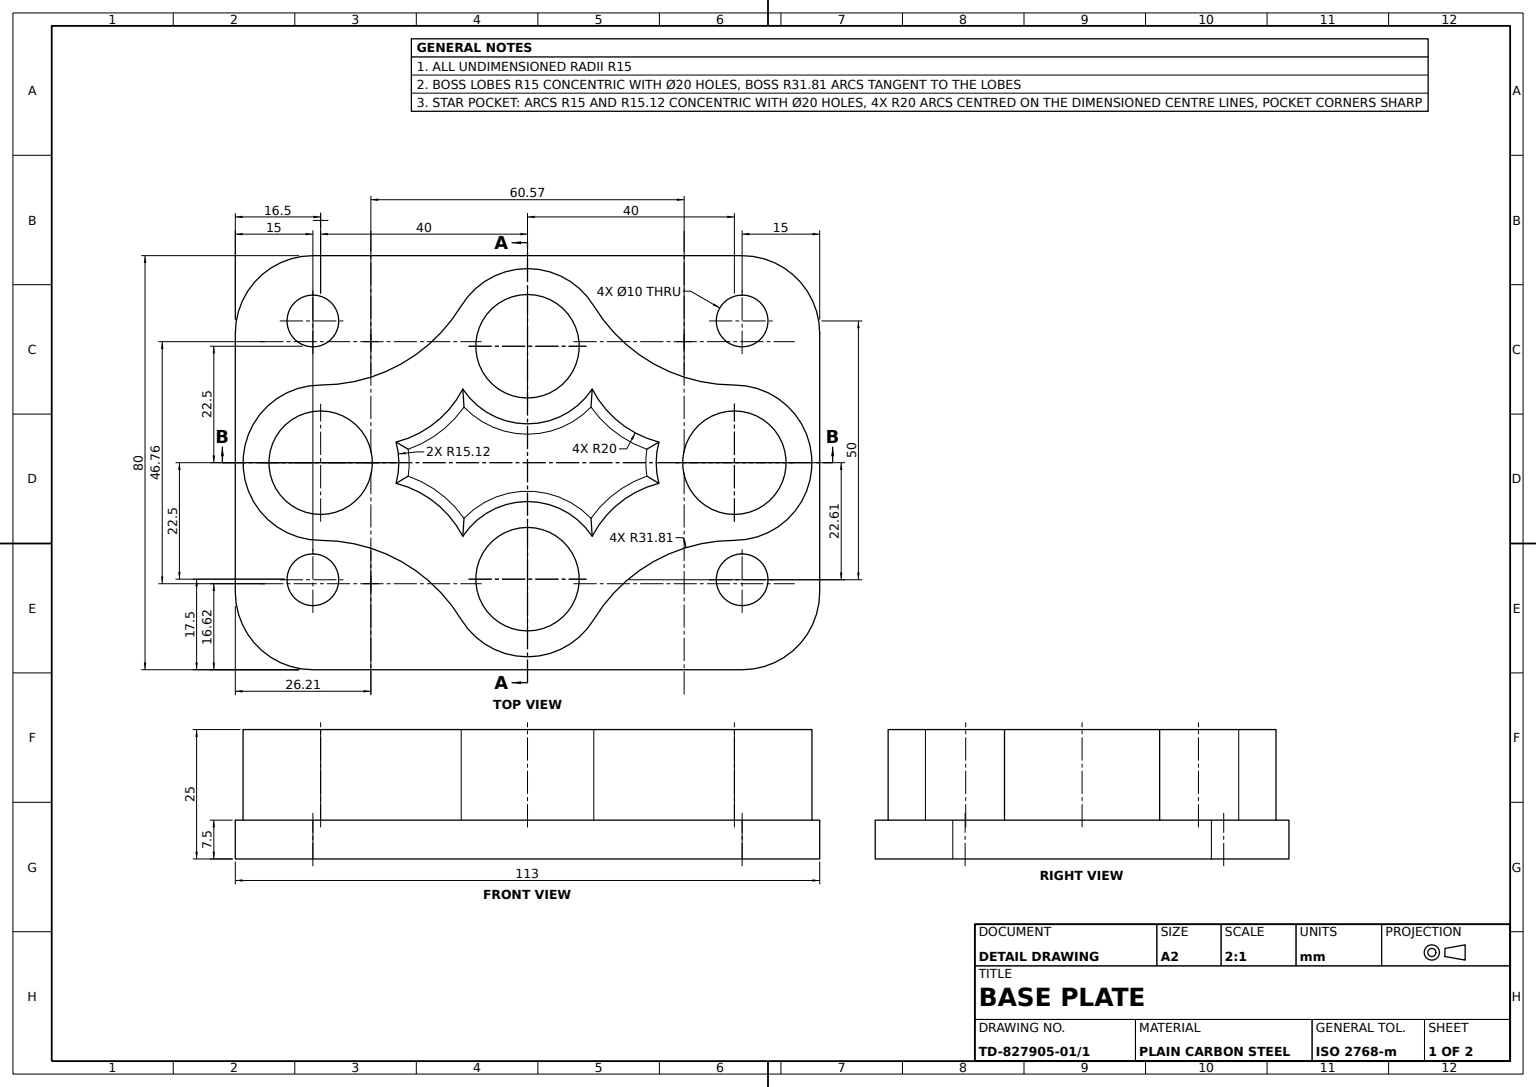
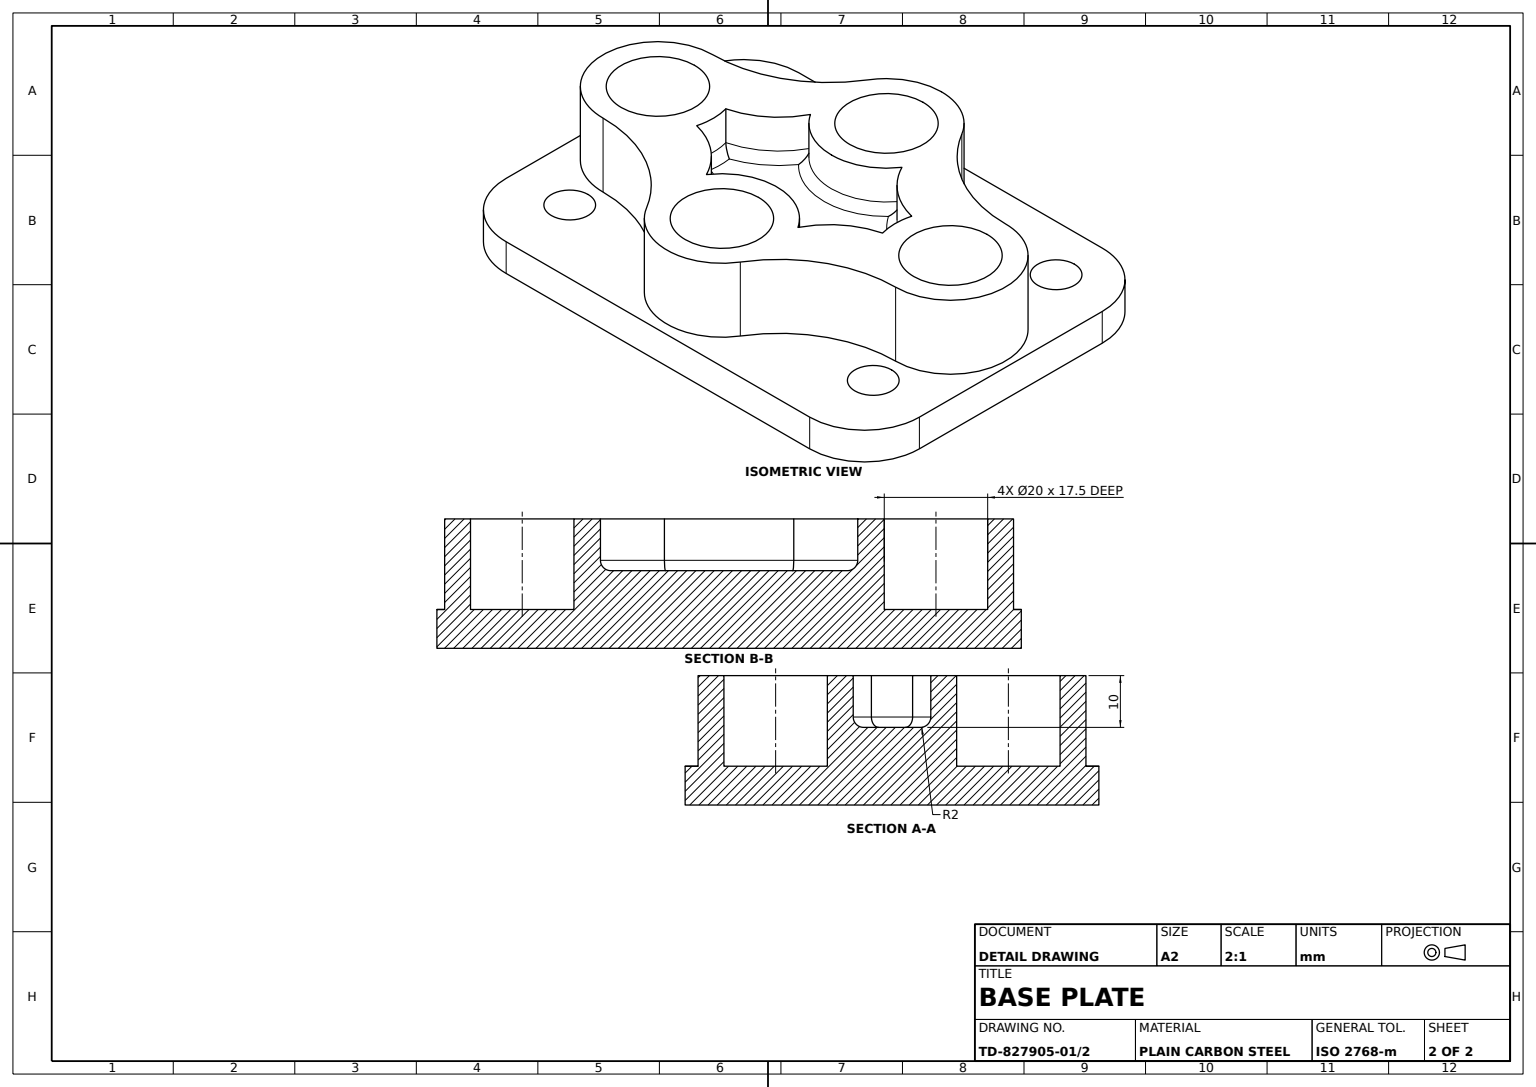
from build123d import *

# Parameters (mm, degrees)
BASE_PLATE_DEPTH           = 3.75
MOUNTING_HOLES_SKETCH_R    = 5
MOUNTING_HOLES_4X_10_DEPTH = 7.5
LOBED_BOSS_DEPTH           = 17.5
STAR_START                 = -10
STAR_POCKET_DEPTH          = 10
BOSS_BORES_SKETCH_R        = 10
BOSS_BORES_4X_DEPTH        = 17.5
POCKET_FILLETS_R2_R        = 2


with BuildPart() as part:
    # Base Plate Profile → Base Plate (new, symmetric)
    with BuildSketch(Plane(origin=(0, 0, 0), x_dir=(1, 0, 0), z_dir=(0, 1, 0))):
        with BuildLine():
            Line((41.5, -40), (-41.5, -40))
            ThreePointArc((-41.5, -40), (-52.106601718, -35.606601718), (-56.5, -25))
            Line((-56.5, -25), (-56.5, 25))
            ThreePointArc((-56.5, 25), (-52.106601718, 35.606601718), (-41.5, 40))
            Line((-41.5, 40), (41.5, 40))
            ThreePointArc((41.5, 40), (52.106601718, 35.606601718), (56.5, 25))
            Line((56.5, 25), (56.5, -25))
            ThreePointArc((56.5, -25), (52.106601718, -35.606601718), (41.5, -40))
        make_face()
    extrude(amount=BASE_PLATE_DEPTH, both=True)

    # Mounting Holes Sketch → Mounting Holes 4xØ10 (cut)
    with BuildSketch(Plane(origin=(0, 3.75, 0), x_dir=(1, 0, 0), z_dir=(0, 1, 0))):
        with Locations(Location((-41.5, 27.385128328, 0), (0, 0, 270))):
            Circle(MOUNTING_HOLES_SKETCH_R)
        with Locations(Location((-41.5, -22.614871672, 0), (0, 0, 270))):
            Circle(MOUNTING_HOLES_SKETCH_R)
        with Locations(Location((41.5, -22.614871672, 0), (0, 0, 90))):
            Circle(MOUNTING_HOLES_SKETCH_R)
        with Locations(Location((41.5, 27.385128328, 0), (0, 0, 90))):
            Circle(MOUNTING_HOLES_SKETCH_R)
    extrude(amount=-MOUNTING_HOLES_4X_10_DEPTH, mode=Mode.SUBTRACT)

    # Lobed Boss Profile → Lobed Boss (add)
    with BuildSketch(Plane(origin=(0, 3.75, 0), x_dir=(1, 0, 0), z_dir=(0, 1, 0))):
        with BuildLine():
            ThreePointArc((-40, 15), (-55, 0), (-40, -15))
            ThreePointArc((-40, -15), (-24.406968906, -19.084611389), (-12.818991098, -30.289317507))
            ThreePointArc((-12.818991098, -30.289317507), (0, -37.5), (12.818991098, -30.289317507))
            ThreePointArc((12.818991098, -30.289317507), (24.406968906, -19.084611389), (40, -15))
            ThreePointArc((40, -15), (55, 0), (40, 15))
            ThreePointArc((40, 15), (24.406968906, 19.084611389), (12.818991098, 30.289317507))
            ThreePointArc((12.818991098, 30.289317507), (0, 37.5), (-12.818991098, 30.289317507))
            ThreePointArc((-12.818991098, 30.289317507), (-24.406968906, 19.084611389), (-40, 15))
        make_face()
    extrude(amount=LOBED_BOSS_DEPTH)

    # Star Pocket Profile → Star Pocket (cut)
    with BuildSketch(Plane(origin=(0, 21.25, 0), x_dir=(1, 0, 0), z_dir=(0, 1, 0)).offset(STAR_START)):
        with BuildLine():
            ThreePointArc((-25.409734785, -3.985145132), (-24.875277829, 0), (-25.409734785, 3.985145132))
            ThreePointArc((-25.409734785, 3.985145132), (-17.85640049, 7.713077773), (-12.507806345, 14.220218576))
            ThreePointArc((-12.507806345, 14.220218576), (0, 7.5), (12.507806345, 14.220218576))
            ThreePointArc((12.507806345, 14.220218576), (17.85640049, 7.713077773), (25.409734785, 3.985145132))
            ThreePointArc((25.409734785, 3.985145132), (24.875277829, 0), (25.409734785, -3.985145132))
            ThreePointArc((25.409734785, -3.985145132), (17.85640049, -7.713077773), (12.507806345, -14.220218576))
            ThreePointArc((12.507806345, -14.220218576), (0, -7.5), (-12.507806345, -14.220218576))
            ThreePointArc((-12.507806345, -14.220218576), (-17.85640049, -7.713077773), (-25.409734785, -3.985145132))
        make_face()
    extrude(amount=STAR_POCKET_DEPTH, mode=Mode.SUBTRACT)

    # Boss Bores Sketch → Boss Bores 4x (cut)
    with BuildSketch(Plane(origin=(0, 21.25, 0), x_dir=(1, 0, 0), z_dir=(0, 1, 0))):
        with Locations(Location((40, 0, 0), (0, 0, 270))):
            Circle(BOSS_BORES_SKETCH_R)
        with Locations(Location((0, -22.5, 0), (0, 0, 270))):
            Circle(BOSS_BORES_SKETCH_R)
        with Locations(Location((0, 22.5, 0), (0, 0, 270))):
            Circle(BOSS_BORES_SKETCH_R)
        with Locations(Location((-40, 0, 0), (0, 0, 270))):
            Circle(BOSS_BORES_SKETCH_R)
    extrude(amount=-BOSS_BORES_4X_DEPTH, mode=Mode.SUBTRACT)

    # Pocket Fillets R2
    pocket_fillets_r2_edges = [part.edges().sort_by_distance(p)[0] for p in [
        (-17.85640049, 11.25, 7.713077773),
        (-24.875277829, 11.25, 0),
        (-17.85640049, 11.25, -7.713077773),
        (0, 11.25, -7.5),
        (17.85640049, 11.25, -7.713077773),
        (24.875277829, 11.25, 0),
        (17.85640049, 11.25, 7.713077773),
        (0, 11.25, 7.5),
    ]]
    fillet(pocket_fillets_r2_edges, radius=POCKET_FILLETS_R2_R)


solid = part.part
